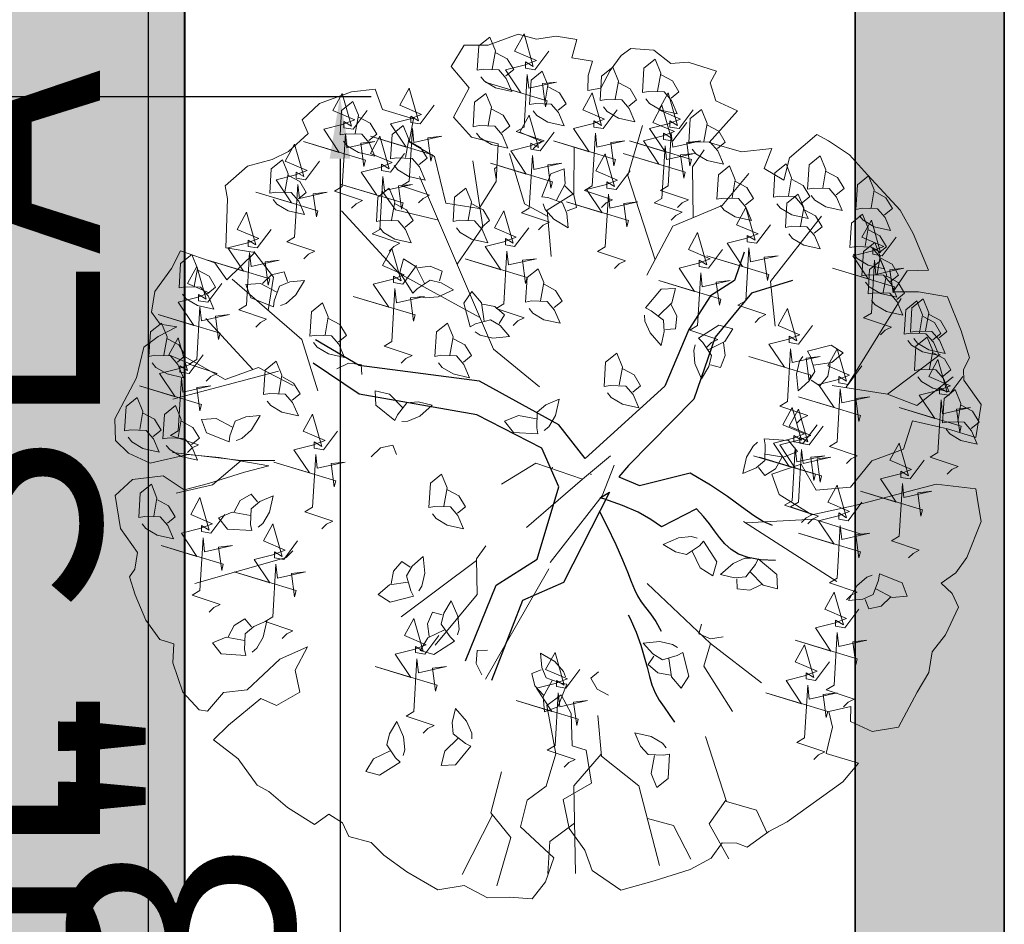
# Model space of a CAD drawing. Units: inches. Extents: x 2337 to 3570, y 1258 to 1938.
# Tile 16 of 30: x 2866 to 2906, y 1722 to 1758. Entities that reach past the tile are written whole.
import ezdxf

# ---------------------------------------------------------------- set-up
doc = ezdxf.new("R2010")
doc.units = ezdxf.units.IN
for name, color, linetype, lineweight in [('A-ANNO-DIMS', 2, 'Continuous', 18), ('A-WALL', 7, 'Continuous', 40), ('ARBOL', 74, 'Continuous', 13), ('C-PROP', 7, 'Continuous', 35)]:
    doc.layers.add(name, color=color, linetype=linetype, lineweight=lineweight)
doc.layers.add('A-WALL-PATT', color=18, linetype='Continuous', lineweight=13, true_color=0x000000)
doc.layers.add('C-PROP-PATT', color=251, linetype='Continuous', lineweight=13, true_color=0x636466)
doc.layers.add('TALLO', color=36, linetype='Continuous')
doc.styles.get("Standard").update_dxf_attribs({"font": 'arial.ttf'})
doc.dimstyles.new('ISO-25', dxfattribs={"dimtxt": 9, "dimasz": 2.5, "dimexe": 1.25, "dimexo": 0.625, "dimtad": 1, "dimdec": 1, "dimlunit": 3, "dimtxsty": 'Standard', "dimcen": 2.5, "dimadec": 0, "dimazin": 0, "dimtfac": 1, "dimtdec": 1, "dimtmove": 0, "dimatfit": 3, "dimfxl": 1, "dimarcsym": 0})

# ---------------------------------------------------------------- blocks, each defined once
blk = doc.blocks.new('fresno')
at = {"layer": 'ARBOL'}
for p, q in [((2.96, 0.991), (3.575, 1.984)), ((-3.638, 1.194), (-4.164, 1.76)), ((-1.151, -0.932), (-1.99, -1.556)), ((-0.974, -3.757), (-1.31, -4.423))]:
    blk.add_line(p, q, dxfattribs=at)
blk.add_lwpolyline([(0.823, 4.745), (0.566, 4.764), (0.459, 4.687), (0.336, 4.518), (0.233, 4.322), (0.087, 4.298), (0.091, 4.464), (0.14, 4.621), (-0.09, 4.659), (-0.033, 4.863), (-0.264, 4.901), (-0.483, 4.866), (-0.686, 4.924), (-1.021, 4.801), (-1.288, 4.8), (-1.431, 4.563), (-1.234, 4.327), (-1.406, 4), (-1.205, 3.778), (-0.909, 3.705), (-0.931, 3.283), (-1.122, 2.983), (-1.491, 3.043), (-1.619, 3.562), (-1.9, 3.727), (-1.851, 3.982), (-2.197, 4.084), (-2.278, 4.31), (-2.543, 4.283), (-2.896, 4.152), (-3.091, 3.971), (-3.022, 3.817), (-3.244, 3.617), (-3.424, 3.528), (-3.697, 3.455), (-3.946, 3.236), (-3.922, 3.09), (-3.94, 2.548), (-3.617, 2.495), (-3.927, 2.19), (-4.062, 2.379), (-4.443, 2.512), (-4.546, 2.316), (-4.73, 2.062), (-4.767, 1.832), (-4.671, 1.698), (-4.486, 1.667), (-4.693, 1.559), (-4.854, 1.444), (-4.934, 1.102), (-5.037, 0.905), (-5.175, 0.644), (-5.166, 0.406), (-5.024, 0.264), (-4.781, 0.153), (-4.363, 0.249), (-4.014, 0.215), (-3.783, 0.177), (-3.46, 0.124), (-3.733, 0.051), (-4.132, -0.073), (-4.404, -0.146), (-4.639, 0.011), (-4.977, -0.028), (-5.172, -0.209), (-5.113, -0.574), (-4.921, -0.843), (-4.951, -1.027), (-5.012, -1.112), (-4.95, -1.311), (-4.83, -1.592), (-4.676, -1.807), (-4.518, -1.856), (-4.529, -2.068), (-4.417, -2.394), (-4.236, -2.59), (-4.143, -2.605), (-3.967, -2.397), (-3.703, -2.37), (-3.339, -2.027), (-3.032, -1.889), (-3.169, -2.15), (-3.115, -2.396), (-3.376, -2.542), (-3.552, -2.466), (-3.909, -2.762), (-4.077, -2.924), (-3.804, -3.135), (-3.592, -3.43), (-3.461, -3.499), (-3.253, -3.676), (-2.953, -3.867), (-2.792, -3.752), (-2.642, -3.848), (-2.572, -4.001), (-2.323, -4.066), (-2.18, -4.208), (-1.926, -4.392), (-1.58, -4.591), (-1.288, -4.545), (-1.027, -4.683), (-0.788, -4.675), (-0.531, -4.693), (-0.382, -4.505), (-0.29, -4.236), (-0.66, -3.891), (-0.588, -3.595), (-0.374, -3.441), (-0.267, -3.079), (-0.368, -2.541), (-0.208, -2.426), (-0.099, -2.633), (-0.087, -2.991), (0.071, -3.04), (0.129, -3.405), (-0.185, -3.59), (-0.119, -3.909), (0.055, -4.151), (0.136, -4.377), (0.456, -4.596), (0.828, -4.491), (1.227, -4.368), (1.461, -4.241), (1.583, -4.071), (1.748, -4.075), (1.86, -4.117), (2.101, -3.944), (2.308, -3.836), (2.925, -3.393), (3.101, -3.185), (2.74, -3.078), (2.812, -2.782), (2.769, -2.61), (3.015, -2.555), (3.012, -2.721), (3.254, -2.832), (3.546, -2.785), (3.752, -2.393), (3.882, -2.177), (3.92, -1.947), (4.069, -1.758), (4.214, -1.451), (4.144, -1.297), (4.021, -1.182), (4.182, -1.067), (4.304, -0.897), (4.464, -0.497), (4.429, -0.279), (4.406, -0.133), (3.964, -0.083), (3.074, -0.315), (2.582, -0.424), (2.217, -0.197), (2.136, 0.029), (2.462, 0.141), (2.628, -0.147), (3.012, -0.116), (3.249, 0.177), (3.602, 0.308), (3.701, 0.623), (4.089, 0.535), (4.404, 0.436), (4.464, 0.805), (4.272, 1.074), (4.267, 1.193), (4.336, 1.324), (4.243, 1.623), (4.092, 2.003), (3.769, 2.057), (3.485, 2.056), (3.642, 2.291), (3.88, 2.299), (3.71, 2.706), (3.563, 2.967), (3.201, 3.358), (3.001, 3.581), (2.766, 3.738), (2.635, 3.807), (2.332, 3.549), (2.268, 3.299), (2.052, 3.429), (2.136, 3.652), (1.798, 3.613), (1.437, 3.72), (1.755, 4.071), (1.513, 4.182), (1.451, 4.381), (1.519, 4.512), (1.204, 4.611), (1.012, 4.596)], close=True, dxfattribs=at)
for points in [[(-1.104, 4.45), (-1.063, 4.399), (-0.939, 4.325), (-0.757, 4.285), (-0.82, 4.431), (-0.903, 4.527), (-1.075, 4.533), (-1.143, 4.521), (-1.126, 4.792), (-1.002, 4.891), (-0.939, 4.738), (-0.975, 4.535)], [(-0.346, 4.735), (-0.501, 4.528), (-0.605, 4.545), (-0.605, 4.614), (-0.519, 4.563), (-0.622, 4.925), (-0.726, 4.735), (-0.484, 4.632), (-0.622, 4.58), (-0.829, 4.528), (-0.657, 4.27), (-1.053, 4.39), (-0.363, 4.183), (-0.381, 4.114), (-0.415, 4.373), (-0.26, 4.39), (-0.57, 4.321), (-0.588, 4.476), (-0.622, 3.89), (-0.708, 3.839), (-0.398, 3.735), (-0.467, 3.701), (-0.519, 3.649)], [(-0.935, 4.717), (-0.809, 4.65), (-0.736, 4.529), (-0.824, 4.459)], [(0.734, 4.203), (0.775, 4.152), (0.9, 4.078), (1.082, 4.038), (1.018, 4.185), (0.936, 4.281), (0.763, 4.287), (0.696, 4.274), (0.712, 4.546), (0.837, 4.645), (0.899, 4.491), (0.863, 4.289)], [(-0.521, 4.069), (-0.48, 4.018), (-0.356, 3.944), (-0.174, 3.904), (-0.237, 4.051), (-0.32, 4.146), (-0.492, 4.152), (-0.56, 4.14), (-0.543, 4.411), (-0.419, 4.511), (-0.356, 4.357), (-0.392, 4.154)], [(0.263, 4.114), (0.304, 4.063), (0.429, 3.989), (0.611, 3.948), (0.547, 4.095), (0.465, 4.191), (0.293, 4.197), (0.225, 4.185), (0.242, 4.456), (0.366, 4.555), (0.428, 4.402), (0.393, 4.199)], [(0.904, 4.471), (1.029, 4.404), (1.102, 4.282), (1.015, 4.212)], [(-1.623, 4.132), (-1.778, 3.925), (-1.882, 3.942), (-1.882, 4.011), (-1.795, 3.959), (-1.899, 4.321), (-2.002, 4.132), (-1.761, 4.028), (-1.899, 3.977), (-2.106, 3.925), (-1.933, 3.666), (-2.33, 3.787), (-1.64, 3.58), (-1.657, 3.511), (-1.692, 3.77), (-1.537, 3.787), (-1.847, 3.718), (-1.864, 3.873), (-1.899, 3.287), (-1.985, 3.235), (-1.675, 3.132), (-1.744, 3.097), (-1.795, 3.046)], [(-0.352, 4.337), (-0.226, 4.269), (-0.153, 4.148), (-0.241, 4.078)], [(0.433, 4.381), (0.558, 4.314), (0.631, 4.193), (0.544, 4.122)], [(-2.368, 4.073), (-2.523, 3.866), (-2.627, 3.883), (-2.627, 3.952), (-2.541, 3.9), (-2.644, 4.262), (-2.748, 4.073), (-2.506, 3.969), (-2.644, 3.918), (-2.851, 3.866), (-2.679, 3.607), (-3.075, 3.728), (-2.385, 3.521), (-2.403, 3.452), (-2.437, 3.711), (-2.282, 3.728), (-2.592, 3.659), (-2.61, 3.814), (-2.644, 3.228), (-2.73, 3.176), (-2.42, 3.073), (-2.489, 3.038), (-2.541, 2.987)], [(-2.629, 3.733), (-2.588, 3.682), (-2.463, 3.608), (-2.281, 3.568), (-2.345, 3.715), (-2.427, 3.81), (-2.6, 3.816), (-2.667, 3.804), (-2.651, 4.075), (-2.526, 4.175), (-2.464, 4.021), (-2.5, 3.818)], [(-1.149, 3.822), (-1.108, 3.771), (-0.983, 3.697), (-0.802, 3.657), (-0.865, 3.804), (-0.948, 3.9), (-1.12, 3.906), (-1.188, 3.893), (-1.171, 4.165), (-1.047, 4.264), (-0.984, 4.111), (-1.02, 3.908)], [(0.413, 4.08), (0.258, 3.873), (0.154, 3.89), (0.154, 3.959), (0.241, 3.908), (0.137, 4.27), (0.034, 4.08), (0.275, 3.977), (0.137, 3.925), (-0.07, 3.873), (0.103, 3.614), (-0.294, 3.735), (0.396, 3.528), (0.379, 3.459), (0.344, 3.718), (0.499, 3.735), (0.189, 3.666), (0.172, 3.821), (0.137, 3.235), (0.051, 3.183), (0.361, 3.08), (0.292, 3.046), (0.241, 2.994)], [(1.259, 4.08), (1.103, 3.873), (1, 3.89), (1, 3.959), (1.086, 3.908), (0.982, 4.27), (0.879, 4.08), (1.12, 3.977), (0.982, 3.925), (0.775, 3.873), (0.948, 3.614), (0.551, 3.735), (1.241, 3.528), (1.224, 3.459), (1.189, 3.718), (1.345, 3.735), (1.034, 3.666), (1.017, 3.821), (0.982, 3.235), (0.896, 3.183), (1.207, 3.08), (1.138, 3.046), (1.086, 2.994)], [(-0.98, 4.09), (-0.854, 4.023), (-0.781, 3.901), (-0.869, 3.831)], [(1.189, 3.942), (1.034, 3.735), (0.931, 3.752), (0.931, 3.821), (1.017, 3.77), (0.913, 4.132), (0.81, 3.942), (1.051, 3.839), (0.913, 3.787), (0.706, 3.735), (0.879, 3.477), (0.482, 3.597), (1.172, 3.39), (1.155, 3.321), (1.12, 3.58), (1.276, 3.597), (0.965, 3.528), (0.948, 3.683), (0.913, 3.097), (0.827, 3.046), (1.138, 2.942), (1.069, 2.908), (1.017, 2.856)], [(1.25, 3.643), (1.291, 3.592), (1.416, 3.518), (1.597, 3.478), (1.534, 3.625), (1.451, 3.721), (1.279, 3.727), (1.211, 3.714), (1.228, 3.985), (1.352, 4.085), (1.415, 3.931), (1.379, 3.729)], [(-2.459, 4), (-2.334, 3.933), (-2.261, 3.812), (-2.348, 3.742)], [(-0.287, 3.833), (-0.442, 3.626), (-0.546, 3.643), (-0.546, 3.712), (-0.46, 3.661), (-0.563, 4.023), (-0.667, 3.833), (-0.425, 3.73), (-0.563, 3.678), (-0.77, 3.626), (-0.598, 3.367), (-0.995, 3.488), (-0.304, 3.281), (-0.322, 3.212), (-0.356, 3.471), (-0.201, 3.488), (-0.511, 3.419), (-0.529, 3.574), (-0.563, 2.988), (-0.649, 2.936), (-0.339, 2.833), (-0.408, 2.799), (-0.46, 2.747)], [(-2.068, 3.464), (-2.027, 3.413), (-1.903, 3.339), (-1.721, 3.299), (-1.784, 3.446), (-1.867, 3.542), (-2.039, 3.547), (-2.107, 3.535), (-2.09, 3.806), (-1.966, 3.906), (-1.903, 3.752), (-1.939, 3.55)], [(0.837, 2.414), (0.533, 3.352), (0.697, 3.906)], [(1.419, 3.911), (1.545, 3.844), (1.618, 3.722), (1.53, 3.652)], [(-1.951, 3.597), (-2.106, 3.39), (-2.209, 3.408), (-2.209, 3.477), (-2.123, 3.425), (-2.227, 3.787), (-2.33, 3.597), (-2.089, 3.494), (-2.227, 3.442), (-2.434, 3.39), (-2.261, 3.132), (-2.658, 3.252), (-1.968, 3.046), (-1.985, 2.977), (-2.02, 3.235), (-1.864, 3.252), (-2.175, 3.183), (-2.192, 3.339), (-2.227, 2.752), (-2.313, 2.701), (-2.002, 2.597), (-2.071, 2.563), (-2.123, 2.511)], [(-1.899, 3.732), (-1.773, 3.664), (-1.7, 3.543), (-1.788, 3.473)], [(-2.898, 3.511), (-3.053, 3.304), (-3.157, 3.321), (-3.157, 3.39), (-3.071, 3.339), (-3.174, 3.701), (-3.278, 3.511), (-3.036, 3.408), (-3.174, 3.356), (-3.381, 3.304), (-3.209, 3.046), (-3.605, 3.166), (-2.915, 2.959), (-2.932, 2.89), (-2.967, 3.149), (-2.812, 3.166), (-3.122, 3.097), (-3.14, 3.253), (-3.174, 2.666), (-3.26, 2.615), (-2.95, 2.511), (-3.019, 2.477), (-3.071, 2.425)], [(-0.063, 3.671), (-0.069, 3.151), (-0.364, 2.965), (-0.319, 2.449)], [(1.259, 2.882), (1.254, 3.446), (1.381, 3.636)], [(-3.413, 3.083), (-3.373, 3.032), (-3.248, 2.958), (-3.066, 2.918), (-3.129, 3.065), (-3.212, 3.161), (-3.384, 3.167), (-3.452, 3.154), (-3.435, 3.425), (-3.311, 3.525), (-3.248, 3.371), (-3.284, 3.169)], [(-1.367, 2.367), (-1.081, 2.78), (-1.193, 3.514)], [(-0.358, 2.895), (-0.615, 3.037), (-0.783, 3.596)], [(0.558, 3.402), (0.403, 3.195), (0.299, 3.212), (0.299, 3.281), (0.386, 3.23), (0.282, 3.592), (0.179, 3.402), (0.42, 3.299), (0.282, 3.247), (0.075, 3.195), (0.248, 2.936), (-0.149, 3.057), (0.541, 2.85), (0.524, 2.781), (0.489, 3.04), (0.644, 3.057), (0.334, 2.988), (0.317, 3.143), (0.282, 2.557), (0.196, 2.505), (0.506, 2.402), (0.437, 2.368), (0.386, 2.316)], [(2.573, 3.128), (2.613, 3.077), (2.738, 3.003), (2.92, 2.963), (2.857, 3.11), (2.774, 3.205), (2.602, 3.211), (2.534, 3.199), (2.551, 3.47), (2.675, 3.57), (2.738, 3.416), (2.702, 3.214)], [(-0.923, 3.449), (-0.951, 3.425), (-0.93, 3.313)], [(-0.41, 3.035), (-0.387, 2.974), (-0.291, 2.865), (-0.131, 2.771), (-0.146, 2.93), (-0.195, 3.047), (-0.357, 3.106), (-0.425, 3.115), (-0.325, 3.368), (-0.176, 3.424), (-0.164, 3.258), (-0.261, 3.077)], [(1.564, 3.016), (1.605, 2.965), (1.729, 2.891), (1.911, 2.851), (1.848, 2.998), (1.765, 3.094), (1.593, 3.099), (1.525, 3.087), (1.542, 3.358), (1.666, 3.458), (1.729, 3.304), (1.693, 3.102)], [(2.191, 3.038), (2.232, 2.987), (2.357, 2.913), (2.539, 2.873), (2.475, 3.02), (2.393, 3.116), (2.221, 3.122), (2.153, 3.109), (2.17, 3.381), (2.294, 3.48), (2.356, 3.326), (2.321, 3.124)], [(-3.244, 3.351), (-3.118, 3.284), (-3.045, 3.162), (-3.133, 3.092)], [(-0.448, 1), (-0.961, 1.419), (-1.784, 3.341)], [(0.746, 2.242), (1.034, 2.786), (1.584, 3.019), (1.879, 3.374)], [(2.361, 3.306), (2.486, 3.239), (2.559, 3.117), (2.472, 3.047)], [(2.742, 3.396), (2.868, 3.328), (2.941, 3.207), (2.853, 3.137)], [(3.111, 2.904), (3.152, 2.853), (3.276, 2.779), (3.458, 2.739), (3.395, 2.886), (3.312, 2.981), (3.14, 2.987), (3.072, 2.975), (3.089, 3.246), (3.213, 3.346), (3.276, 3.192), (3.24, 2.99)], [(-2.225, 2.77), (-2.184, 2.718), (-2.06, 2.645), (-1.878, 2.604), (-1.941, 2.751), (-2.024, 2.847), (-2.196, 2.853), (-2.264, 2.84), (-2.247, 3.112), (-2.123, 3.211), (-2.06, 3.058), (-2.096, 2.855)], [(-1.575, 2.854), (-2.052, 2.969), (-2.2, 3.178)], [(-1.373, 2.77), (-1.332, 2.718), (-1.208, 2.645), (-1.026, 2.604), (-1.089, 2.751), (-1.172, 2.847), (-1.344, 2.853), (-1.412, 2.84), (-1.395, 3.112), (-1.271, 3.211), (-1.208, 3.058), (-1.244, 2.855)], [(-0.166, 3.238), (-0.068, 3.135), (-0.036, 2.997), (-0.141, 2.957)], [(1.733, 3.284), (1.859, 3.216), (1.932, 3.095), (1.844, 3.025)], [(2.326, 2.702), (2.367, 2.651), (2.492, 2.577), (2.673, 2.537), (2.61, 2.684), (2.527, 2.78), (2.355, 2.786), (2.287, 2.773), (2.304, 3.045), (2.428, 3.144), (2.491, 2.99), (2.455, 2.788)], [(3.28, 3.172), (3.406, 3.104), (3.479, 2.983), (3.391, 2.913)], [(-2.056, 3.037), (-1.93, 2.97), (-1.857, 2.849), (-1.945, 2.778)], [(-0.57, 2.77), (-0.726, 2.563), (-0.829, 2.58), (-0.829, 2.649), (-0.743, 2.597), (-0.846, 2.959), (-0.95, 2.77), (-0.708, 2.666), (-0.846, 2.615), (-1.053, 2.563), (-0.881, 2.304), (-1.278, 2.425), (-0.588, 2.218), (-0.605, 2.149), (-0.639, 2.408), (-0.484, 2.425), (-0.795, 2.356), (-0.812, 2.511), (-0.846, 1.925), (-0.933, 1.873), (-0.622, 1.77), (-0.691, 1.735), (-0.743, 1.684)], [(-1.204, 3.037), (-1.078, 2.97), (-1.005, 2.849), (-1.093, 2.778)], [(2.121, 2.804), (1.966, 2.597), (1.862, 2.615), (1.862, 2.683), (1.949, 2.632), (1.845, 2.994), (1.742, 2.804), (1.983, 2.701), (1.845, 2.649), (1.638, 2.597), (1.811, 2.339), (1.414, 2.459), (2.104, 2.252), (2.087, 2.184), (2.052, 2.442), (2.207, 2.459), (1.897, 2.39), (1.88, 2.546), (1.845, 1.959), (1.759, 1.908), (2.069, 1.804), (2, 1.77), (1.949, 1.718)], [(2.495, 2.97), (2.621, 2.903), (2.694, 2.781), (2.606, 2.711)], [(-3.434, 2.752), (-3.59, 2.546), (-3.693, 2.563), (-3.693, 2.632), (-3.607, 2.58), (-3.71, 2.942), (-3.814, 2.752), (-3.572, 2.649), (-3.71, 2.597), (-3.917, 2.546), (-3.745, 2.287), (-4.142, 2.408), (-3.452, 2.201), (-3.469, 2.132), (-3.503, 2.39), (-3.348, 2.408), (-3.659, 2.339), (-3.676, 2.494), (-3.71, 1.908), (-3.797, 1.856), (-3.486, 1.753), (-3.555, 1.718), (-3.607, 1.666)], [(-1.112, 1.773), (-2.014, 2.265), (-2.654, 2.957)], [(2.171, 1.674), (2.121, 2.172), (2.689, 2.898)], [(3.519, 2.666), (3.363, 2.459), (3.26, 2.477), (3.26, 2.546), (3.346, 2.494), (3.243, 2.856), (3.139, 2.666), (3.381, 2.563), (3.243, 2.511), (3.036, 2.459), (3.208, 2.201), (2.811, 2.321), (3.501, 2.115), (3.484, 2.046), (3.45, 2.304), (3.605, 2.321), (3.294, 2.252), (3.277, 2.408), (3.243, 1.821), (3.156, 1.77), (3.467, 1.666), (3.398, 1.632), (3.346, 1.58)], [(3.043, 2.478), (3.084, 2.427), (3.209, 2.353), (3.391, 2.313), (3.327, 2.46), (3.245, 2.556), (3.073, 2.562), (3.005, 2.549), (3.022, 2.82), (3.146, 2.92), (3.208, 2.766), (3.173, 2.564)], [(3.213, 2.746), (3.338, 2.679), (3.411, 2.557), (3.324, 2.487)], [(1.586, 2.528), (1.431, 2.321), (1.327, 2.339), (1.327, 2.408), (1.414, 2.356), (1.31, 2.718), (1.207, 2.528), (1.448, 2.425), (1.31, 2.373), (1.103, 2.321), (1.276, 2.063), (0.879, 2.184), (1.569, 1.977), (1.552, 1.908), (1.517, 2.166), (1.673, 2.184), (1.362, 2.115), (1.345, 2.27), (1.31, 1.684), (1.224, 1.632), (1.535, 1.528), (1.466, 1.494), (1.414, 1.442)], [(-1.817, 2.351), (-1.972, 2.144), (-2.075, 2.162), (-2.075, 2.231), (-1.989, 2.179), (-2.093, 2.541), (-2.196, 2.351), (-1.955, 2.248), (-2.093, 2.196), (-2.3, 2.144), (-2.127, 1.886), (-2.524, 2.006), (-1.834, 1.8), (-1.851, 1.731), (-1.886, 1.989), (-1.73, 2.006), (-2.041, 1.937), (-2.058, 2.093), (-2.093, 1.506), (-2.179, 1.455), (-1.868, 1.351), (-1.937, 1.317), (-1.989, 1.265)], [(3.178, 2.165), (3.219, 2.113), (3.344, 2.04), (3.525, 1.999), (3.462, 2.146), (3.379, 2.242), (3.207, 2.248), (3.139, 2.236), (3.156, 2.507), (3.28, 2.606), (3.343, 2.453), (3.307, 2.25)], [(-4.422, 2.03), (-4.381, 1.979), (-4.257, 1.905), (-4.075, 1.865), (-4.138, 2.012), (-4.221, 2.108), (-4.393, 2.114), (-4.461, 2.101), (-4.444, 2.372), (-4.32, 2.472), (-4.257, 2.318), (-4.293, 2.116)], [(-3.468, 1.85), (-3.409, 2.222), (-3.628, 2.505)], [(-1.786, 2.007), (-1.722, 1.99), (-1.578, 2.003), (-1.407, 2.078), (-1.545, 2.159), (-1.668, 2.188), (-1.811, 2.092), (-1.859, 2.042), (-2.004, 2.271), (-1.962, 2.425), (-1.821, 2.337), (-1.731, 2.152)], [(3.347, 2.432), (3.473, 2.365), (3.546, 2.244), (3.458, 2.173)], [(-3.986, 2.149), (-4.142, 1.942), (-4.245, 1.959), (-4.245, 2.028), (-4.159, 1.977), (-4.262, 2.339), (-4.366, 2.149), (-4.124, 2.046), (-4.262, 1.994), (-4.47, 1.942), (-4.297, 1.684), (-4.694, 1.804), (-4.004, 1.597), (-4.021, 1.528), (-4.055, 1.787), (-3.9, 1.804), (-4.211, 1.735), (-4.228, 1.89), (-4.262, 1.304), (-4.349, 1.253), (-4.038, 1.149), (-4.107, 1.115), (-4.159, 1.063)], [(-1.806, 2.323), (-1.665, 2.343), (-1.534, 2.287), (-1.564, 2.179)], [(-0.566, 1.873), (-0.525, 1.822), (-0.4, 1.748), (-0.219, 1.708), (-0.282, 1.855), (-0.365, 1.951), (-0.537, 1.957), (-0.605, 1.944), (-0.588, 2.216), (-0.464, 2.315), (-0.401, 2.162), (-0.437, 1.959)], [(3.245, 1.963), (3.286, 1.912), (3.411, 1.838), (3.593, 1.798), (3.529, 1.945), (3.447, 2.041), (3.274, 2.046), (3.206, 2.034), (3.223, 2.305), (3.347, 2.405), (3.41, 2.251), (3.374, 2.049)], [(-4.253, 2.298), (-4.127, 2.231), (-4.054, 2.109), (-4.142, 2.039)], [(-2.916, 0.958), (-3.096, 1.528), (-3.871, 2.197)], [(-3.533, 2.149), (-3.43, 2.247), (-3.292, 2.279), (-3.252, 2.174)], [(3.415, 2.231), (3.54, 2.163), (3.613, 2.042), (3.525, 1.972)], [(-3.331, 1.905), (-3.269, 1.928), (-3.161, 2.024), (-3.066, 2.184), (-3.226, 2.169), (-3.342, 2.121), (-3.401, 1.958), (-3.41, 1.89), (-3.663, 1.99), (-3.719, 2.139), (-3.554, 2.151), (-3.372, 2.054)], [(-0.397, 2.141), (-0.271, 2.074), (-0.198, 1.952), (-0.286, 1.882)], [(0.72, 1.798), (0.723, 1.733), (0.781, 1.6), (0.904, 1.46), (0.939, 1.616), (0.929, 1.742), (0.793, 1.848), (0.73, 1.878), (0.904, 2.088), (1.062, 2.095), (1.023, 1.934), (0.875, 1.791)], [(-1.164, 1.612), (-1.109, 1.576), (-0.967, 1.544), (-0.782, 1.562), (-0.888, 1.682), (-0.996, 1.748), (-1.162, 1.7), (-1.222, 1.667), (-1.29, 1.93), (-1.203, 2.063), (-1.096, 1.937), (-1.067, 1.733)], [(3.716, 1.537), (3.757, 1.486), (3.882, 1.412), (4.063, 1.372), (4, 1.519), (3.917, 1.615), (3.745, 1.621), (3.677, 1.608), (3.694, 1.88), (3.818, 1.979), (3.881, 1.825), (3.845, 1.623)], [(-2.965, 1.493), (-2.924, 1.441), (-2.799, 1.368), (-2.618, 1.327), (-2.681, 1.474), (-2.764, 1.57), (-2.936, 1.576), (-3.004, 1.564), (-2.987, 1.835), (-2.863, 1.934), (-2.8, 1.781), (-2.836, 1.578)], [(-1.085, 1.919), (-0.945, 1.893), (-0.838, 1.801), (-0.9, 1.707)], [(1.014, 1.915), (1.077, 1.787), (1.064, 1.646), (0.952, 1.64)], [(2.587, 1.684), (2.432, 1.477), (2.328, 1.494), (2.328, 1.563), (2.414, 1.511), (2.311, 1.873), (2.207, 1.684), (2.449, 1.58), (2.311, 1.528), (2.104, 1.477), (2.276, 1.218), (1.88, 1.339), (2.57, 1.132), (2.552, 1.063), (2.518, 1.321), (2.673, 1.339), (2.363, 1.27), (2.345, 1.425), (2.311, 0.839), (2.225, 0.787), (2.535, 0.684), (2.466, 0.649), (2.414, 0.597)], [(3.649, 1.515), (3.69, 1.464), (3.814, 1.39), (3.996, 1.35), (3.933, 1.497), (3.85, 1.592), (3.678, 1.598), (3.61, 1.586), (3.627, 1.857), (3.751, 1.957), (3.814, 1.803), (3.778, 1.601)], [(-2.796, 1.76), (-2.67, 1.693), (-2.597, 1.572), (-2.685, 1.501)], [(3.818, 1.783), (3.944, 1.715), (4.017, 1.594), (3.929, 1.524)], [(3.885, 1.805), (4.011, 1.738), (4.084, 1.616), (3.996, 1.546)], [(-4.759, 1.269), (-4.718, 1.217), (-4.593, 1.144), (-4.411, 1.103), (-4.475, 1.25), (-4.557, 1.346), (-4.729, 1.352), (-4.797, 1.339), (-4.78, 1.611), (-4.656, 1.71), (-4.594, 1.557), (-4.629, 1.354)], [(-1.575, 1.269), (-1.534, 1.217), (-1.409, 1.144), (-1.228, 1.103), (-1.291, 1.25), (-1.373, 1.346), (-1.546, 1.352), (-1.614, 1.339), (-1.597, 1.611), (-1.473, 1.71), (-1.41, 1.557), (-1.446, 1.354)], [(1.283, 1.469), (1.266, 1.405), (1.279, 1.261), (1.354, 1.09), (1.435, 1.228), (1.464, 1.351), (1.368, 1.494), (1.318, 1.542), (1.547, 1.687), (1.7, 1.645), (1.613, 1.504), (1.428, 1.414)], [(-4.193, 1.356), (-4.349, 1.149), (-4.452, 1.166), (-4.452, 1.235), (-4.366, 1.184), (-4.469, 1.546), (-4.573, 1.356), (-4.331, 1.253), (-4.469, 1.201), (-4.677, 1.149), (-4.504, 0.89), (-4.901, 1.011), (-4.211, 0.804), (-4.228, 0.735), (-4.262, 0.994), (-4.107, 1.011), (-4.418, 0.942), (-4.435, 1.097), (-4.469, 0.511), (-4.556, 0.459), (-4.245, 0.356), (-4.314, 0.322), (-4.366, 0.27)], [(-4.589, 1.536), (-4.464, 1.469), (-4.391, 1.348), (-4.478, 1.277)], [(-1.406, 1.536), (-1.28, 1.469), (-1.207, 1.348), (-1.295, 1.277)], [(3.761, 1.112), (3.802, 1.061), (3.926, 0.987), (4.108, 0.947), (4.045, 1.093), (3.962, 1.189), (3.79, 1.195), (3.722, 1.183), (3.739, 1.454), (3.863, 1.553), (3.926, 1.4), (3.89, 1.197)], [(1.599, 1.489), (1.618, 1.348), (1.563, 1.217), (1.455, 1.247)], [(2.479, 1.34), (2.443, 1.285), (2.411, 1.143), (2.429, 0.958), (2.549, 1.064), (2.615, 1.172), (2.567, 1.338), (2.534, 1.398), (2.797, 1.466), (2.93, 1.379), (2.804, 1.272), (2.6, 1.243)], [(3.139, 1.235), (2.984, 1.028), (2.88, 1.046), (2.88, 1.115), (2.967, 1.063), (2.863, 1.425), (2.759, 1.235), (3.001, 1.132), (2.863, 1.08), (2.656, 1.028), (2.828, 0.77), (2.432, 0.891), (3.122, 0.684), (3.105, 0.615), (3.07, 0.873), (3.225, 0.891), (2.915, 0.822), (2.897, 0.977), (2.863, 0.391), (2.777, 0.339), (3.087, 0.235), (3.018, 0.201), (2.967, 0.149)], [(-3.192, 1.017), (-3.578, 1.215), (-3.949, 1.081), (-4.398, 1.339)], [(0.308, 0.933), (0.349, 0.881), (0.474, 0.807), (0.656, 0.767), (0.592, 0.914), (0.51, 1.01), (0.337, 1.016), (0.27, 1.003), (0.286, 1.275), (0.411, 1.374), (0.473, 1.221), (0.437, 1.018)], [(4.01, 1.36), (3.422, 0.918)], [(3.93, 1.379), (4.056, 1.312), (4.129, 1.191), (4.041, 1.121)], [(-3.481, 0.843), (-3.44, 0.792), (-3.315, 0.718), (-3.133, 0.678), (-3.197, 0.825), (-3.279, 0.92), (-3.451, 0.926), (-3.519, 0.914), (-3.502, 1.185), (-3.378, 1.285), (-3.316, 1.131), (-3.351, 0.928)], [(-2.703, 1.201), (-2.575, 1.263), (-2.433, 1.251), (-2.428, 1.139)], [(2.786, 1.261), (2.76, 1.121), (2.668, 1.014), (2.574, 1.076)], [(4.26, 1.115), (4.105, 0.908), (4.002, 0.925), (4.002, 0.994), (4.088, 0.942), (3.984, 1.304), (3.881, 1.115), (4.122, 1.011), (3.984, 0.959), (3.777, 0.908), (3.95, 0.649), (3.553, 0.77), (4.243, 0.563), (4.226, 0.494), (4.191, 0.753), (4.347, 0.77), (4.036, 0.701), (4.019, 0.856), (3.984, 0.27), (3.898, 0.218), (4.209, 0.115), (4.14, 0.08), (4.088, 0.029)], [(-3.354, 1.176), (-4.529, 0.864)], [(-3.311, 1.111), (-3.186, 1.043), (-3.113, 0.922), (-3.2, 0.852)], [(0.478, 1.2), (0.603, 1.133), (0.676, 1.011), (0.589, 0.941)], [(2.808, 1.015), (3.422, 0.918), (3.422, 0.918), (3.748, 0.794), (4.154, 1.111)], [(-5.028, 0.44), (-4.987, 0.388), (-4.862, 0.315), (-4.68, 0.274), (-4.744, 0.421), (-4.826, 0.517), (-4.998, 0.523), (-5.066, 0.511), (-5.049, 0.782), (-4.925, 0.881), (-4.863, 0.728), (-4.898, 0.525)], [(-1.981, 0.615), (-1.915, 0.618), (-1.782, 0.676), (-1.643, 0.799), (-1.799, 0.834), (-1.925, 0.824), (-2.031, 0.688), (-2.061, 0.626), (-2.27, 0.799), (-2.278, 0.958), (-2.117, 0.918), (-1.974, 0.77)], [(4.075, 0.529), (4.116, 0.478), (4.24, 0.404), (4.422, 0.364), (4.359, 0.511), (4.276, 0.607), (4.104, 0.613), (4.036, 0.6), (4.053, 0.871), (4.177, 0.971), (4.24, 0.817), (4.204, 0.615)], [(-4.602, 0.35), (-4.561, 0.299), (-4.436, 0.225), (-4.254, 0.185), (-4.318, 0.332), (-4.4, 0.428), (-4.572, 0.433), (-4.64, 0.421), (-4.623, 0.692), (-4.499, 0.792), (-4.437, 0.638), (-4.472, 0.436)], [(-0.397, 0.517), (-0.346, 0.557), (-0.272, 0.682), (-0.232, 0.864), (-0.379, 0.801), (-0.474, 0.718), (-0.48, 0.546), (-0.468, 0.478), (-0.739, 0.495), (-0.838, 0.619), (-0.685, 0.682), (-0.482, 0.646)], [(2.639, 0.58), (2.483, 0.373), (2.38, 0.391), (2.38, 0.46), (2.466, 0.408), (2.363, 0.77), (2.259, 0.58), (2.501, 0.477), (2.363, 0.425), (2.156, 0.373), (2.328, 0.115), (1.931, 0.235), (2.621, 0.029), (2.604, -0.04), (2.57, 0.218), (2.725, 0.235), (2.414, 0.166), (2.397, 0.322), (2.363, -0.265), (2.276, -0.316), (2.587, -0.42), (2.518, -0.454), (2.466, -0.506)], [(4.244, 0.797), (4.37, 0.73), (4.443, 0.608), (4.355, 0.538)], [(-4.858, 0.707), (-4.733, 0.64), (-4.66, 0.519), (-4.747, 0.448)], [(-3.824, 0.404), (-3.763, 0.427), (-3.654, 0.523), (-3.559, 0.683), (-3.719, 0.668), (-3.835, 0.62), (-3.894, 0.457), (-3.903, 0.389), (-4.156, 0.489), (-4.212, 0.638), (-4.047, 0.65), (-3.865, 0.553)], [(-2.698, 0.509), (-2.854, 0.302), (-2.957, 0.319), (-2.957, 0.388), (-2.871, 0.336), (-2.974, 0.698), (-3.078, 0.509), (-2.836, 0.405), (-2.974, 0.353), (-3.182, 0.302), (-3.009, 0.043), (-3.406, 0.164), (-2.716, -0.043), (-2.733, -0.112), (-2.767, 0.147), (-2.612, 0.164), (-2.923, 0.095), (-2.94, 0.25), (-2.974, -0.336), (-3.061, -0.388), (-2.75, -0.491), (-2.819, -0.526), (-2.871, -0.577)], [(2.708, 0.563), (2.552, 0.356), (2.449, 0.373), (2.449, 0.442), (2.535, 0.391), (2.432, 0.753), (2.328, 0.563), (2.57, 0.46), (2.432, 0.408), (2.225, 0.356), (2.397, 0.097), (2, 0.218), (2.69, 0.011), (2.673, -0.058), (2.639, 0.201), (2.794, 0.218), (2.483, 0.149), (2.466, 0.304), (2.432, -0.282), (2.345, -0.334), (2.656, -0.437), (2.587, -0.471), (2.535, -0.523)], [(-4.432, 0.618), (-4.307, 0.55), (-4.234, 0.429), (-4.321, 0.359)], [(-2.322, 0.222), (-2.219, 0.321), (-2.081, 0.353), (-2.042, 0.248)], [(1.978, 0.384), (1.927, 0.343), (1.853, 0.218), (1.813, 0.036), (1.96, 0.1), (2.056, 0.182), (2.061, 0.355), (2.049, 0.422), (2.32, 0.406), (2.42, 0.281), (2.266, 0.219), (2.064, 0.254)], [(3.829, 0.184), (3.674, -0.023), (3.57, -0.006), (3.57, 0.063), (3.657, 0.011), (3.553, 0.373), (3.45, 0.184), (3.691, 0.08), (3.553, 0.029), (3.346, -0.023), (3.519, -0.282), (3.122, -0.161), (3.812, -0.368), (3.795, -0.437), (3.76, -0.178), (3.915, -0.161), (3.605, -0.23), (3.588, -0.075), (3.553, -0.661), (3.467, -0.713), (3.777, -0.816), (3.708, -0.851), (3.657, -0.902)], [(-3.394, 0.18), (-3.77, 0.182), (-4.532, 0.27)], [(-0.596, -0.564), (0.03, -0.026), (0.339, 0.235)], [(-3.77, 0.182), (-4.09, -0.088), (-4.494, -0.18)], [(0.03, -0.026), (-0.491, 0.154), (-0.871, -0.08)], [(0.38, 0.131), (0.248, -0.21), (-0.33, -0.951)], [(2.246, 0.214), (2.178, 0.089), (2.057, 0.016), (1.987, 0.103)], [(-1.642, -0.412), (-1.601, -0.463), (-1.477, -0.537), (-1.295, -0.577), (-1.358, -0.43), (-1.441, -0.334), (-1.613, -0.328), (-1.681, -0.341), (-1.664, -0.069), (-1.54, 0.03), (-1.477, -0.124), (-1.513, -0.326)], [(-4.871, -0.524), (-4.83, -0.575), (-4.705, -0.649), (-4.523, -0.689), (-4.587, -0.542), (-4.669, -0.446), (-4.841, -0.44), (-4.909, -0.453), (-4.893, -0.181), (-4.768, -0.082), (-4.706, -0.236), (-4.741, -0.438)], [(3.139, -0.282), (2.984, -0.489), (2.88, -0.471), (2.88, -0.402), (2.967, -0.454), (2.863, -0.092), (2.759, -0.282), (3.001, -0.385), (2.863, -0.437), (2.656, -0.489), (2.828, -0.747), (2.432, -0.627), (3.122, -0.834), (3.105, -0.902), (3.07, -0.644), (3.225, -0.627), (2.915, -0.696), (2.897, -0.54), (2.863, -1.127), (2.777, -1.178), (3.087, -1.282), (3.018, -1.316), (2.967, -1.368)], [(-3.58, -0.559), (-3.529, -0.518), (-3.455, -0.393), (-3.415, -0.211), (-3.562, -0.275), (-3.658, -0.357), (-3.664, -0.53), (-3.651, -0.597), (-3.923, -0.581), (-4.022, -0.456), (-3.868, -0.394), (-3.666, -0.43)], [(-3.848, -0.389), (-3.781, -0.264), (-3.659, -0.191), (-3.589, -0.278)], [(-1.473, -0.144), (-1.347, -0.211), (-1.274, -0.333), (-1.362, -0.403)], [(-4.701, -0.256), (-4.576, -0.323), (-4.503, -0.445), (-4.59, -0.515)], [(-3.952, -0.42), (-4.107, -0.627), (-4.211, -0.609), (-4.211, -0.54), (-4.124, -0.592), (-4.228, -0.23), (-4.331, -0.42), (-4.09, -0.523), (-4.228, -0.575), (-4.435, -0.627), (-4.262, -0.885), (-4.659, -0.765), (-3.969, -0.971), (-3.986, -1.04), (-4.021, -0.782), (-3.866, -0.765), (-4.176, -0.834), (-4.193, -0.678), (-4.228, -1.265), (-4.314, -1.316), (-4.004, -1.42), (-4.073, -1.454), (-4.124, -1.506)], [(-3.141, -0.713), (-3.296, -0.92), (-3.4, -0.902), (-3.4, -0.834), (-3.314, -0.885), (-3.417, -0.523), (-3.521, -0.713), (-3.279, -0.816), (-3.417, -0.868), (-3.624, -0.92), (-3.452, -1.178), (-3.848, -1.058), (-3.158, -1.265), (-3.175, -1.333), (-3.21, -1.075), (-3.055, -1.058), (-3.365, -1.127), (-3.383, -0.971), (-3.417, -1.558), (-3.503, -1.609), (-3.193, -1.713), (-3.262, -1.747), (-3.314, -1.799)], [(1.822, -0.495), (2.859, -1.165)], [(1.846, -0.51), (2.605, -0.469), (3.129, -0.637)], [(-1.047, -0.767), (-1.151, -0.913), (-1.144, -1.307), (-1.61, -1.871)], [(1.304, -0.681), (1.241, -0.664), (1.097, -0.678), (0.926, -0.752), (1.064, -0.833), (1.187, -0.862), (1.33, -0.766), (1.377, -0.716), (1.523, -0.945), (1.481, -1.099), (1.34, -1.011), (1.25, -0.826)], [(-3.195, -0.824), (-3.267, -0.898), (-4.285, -1.185)], [(-1.794, -1.268), (-1.758, -1.214), (-1.726, -1.072), (-1.744, -0.887), (-1.865, -0.993), (-1.93, -1.101), (-1.883, -1.266), (-1.85, -1.327), (-2.113, -1.395), (-2.246, -1.307), (-2.119, -1.2), (-1.916, -1.172)], [(-2.101, -1.19), (-2.076, -1.05), (-1.983, -0.943), (-1.889, -1.004)], [(1.903, -0.903), (1.837, -0.905), (1.704, -0.963), (1.565, -1.086), (1.721, -1.122), (1.847, -1.111), (1.953, -0.975), (1.983, -0.913), (2.192, -1.086), (2.2, -1.245), (2.039, -1.205), (1.896, -1.057)], [(-0.346, -1.024), (-1.05, -2.251)], [(3.253, -1.094), (3.192, -1.117), (3.083, -1.213), (2.988, -1.374), (3.148, -1.359), (3.264, -1.31), (3.323, -1.148), (3.332, -1.079), (3.585, -1.179), (3.641, -1.328), (3.476, -1.34), (3.294, -1.244)], [(0.748, -1.185), (1.452, -1.855), (2.021, -2.292)], [(2.02, -1.197), (1.891, -1.259), (1.75, -1.247), (1.745, -1.134)], [(3.105, -1.471), (2.949, -1.678), (2.846, -1.661), (2.846, -1.592), (2.932, -1.644), (2.829, -1.282), (2.725, -1.471), (2.967, -1.575), (2.829, -1.627), (2.621, -1.678), (2.794, -1.937), (2.397, -1.816), (3.087, -2.023), (3.07, -2.092), (3.036, -1.833), (3.191, -1.816), (2.88, -1.885), (2.863, -1.73), (2.829, -2.316), (2.742, -2.368), (3.053, -2.471), (2.984, -2.506), (2.932, -2.558)], [(-1.361, -1.756), (-1.343, -1.693), (-1.357, -1.548), (-1.431, -1.377), (-1.513, -1.515), (-1.542, -1.638), (-1.445, -1.781), (-1.395, -1.829), (-1.625, -1.974), (-1.778, -1.932), (-1.691, -1.791), (-1.506, -1.701)], [(3.455, -1.338), (3.352, -1.437), (3.214, -1.469), (3.175, -1.364)], [(-1.677, -1.776), (-1.696, -1.635), (-1.641, -1.504), (-1.533, -1.534)], [(-3.648, -1.948), (-3.596, -1.907), (-3.523, -1.782), (-3.482, -1.6), (-3.629, -1.664), (-3.725, -1.746), (-3.731, -1.919), (-3.719, -1.986), (-3.99, -1.97), (-4.089, -1.845), (-3.936, -1.783), (-3.733, -1.819)], [(-3.915, -1.778), (-3.848, -1.653), (-3.727, -1.58), (-3.656, -1.667)], [(-1.571, -1.764), (-1.726, -1.971), (-1.83, -1.954), (-1.83, -1.885), (-1.744, -1.937), (-1.847, -1.575), (-1.951, -1.764), (-1.709, -1.868), (-1.847, -1.92), (-2.054, -1.971), (-1.882, -2.23), (-2.278, -2.109), (-1.588, -2.316), (-1.605, -2.385), (-1.64, -2.127), (-1.485, -2.109), (-1.795, -2.178), (-1.813, -2.023), (-1.847, -2.609), (-1.933, -2.661), (-1.623, -2.764), (-1.692, -2.799), (-1.744, -2.851)], [(1.593, -1.781), (1.452, -1.801), (1.322, -1.746), (1.352, -1.637)], [(1.086, -1.899), (1.031, -1.863), (0.89, -1.831), (0.704, -1.849), (0.81, -1.969), (0.918, -2.035), (1.084, -1.987), (1.145, -1.954), (1.212, -2.218), (1.125, -2.35), (1.018, -2.224), (0.989, -2.02)], [(1.452, -1.855), (1.379, -2.105), (1.698, -2.609)], [(-1.092, -2.202), (-1.154, -2.074), (-1.142, -1.933), (-1.03, -1.928)], [(-0.001, -2.144), (-0.156, -2.351), (-0.26, -2.333), (-0.26, -2.264), (-0.174, -2.316), (-0.277, -1.954), (-0.381, -2.144), (-0.139, -2.247), (-0.277, -2.299), (-0.484, -2.351), (-0.312, -2.609), (-0.708, -2.489), (-0.018, -2.695), (-0.035, -2.764), (-0.07, -2.506), (0.085, -2.489), (-0.225, -2.558), (-0.243, -2.402), (-0.277, -2.989), (-0.363, -3.04), (-0.053, -3.144), (-0.122, -3.178), (-0.174, -3.23)], [(-0.161, -2.225), (-0.184, -2.163), (-0.28, -2.055), (-0.44, -1.96), (-0.425, -2.12), (-0.376, -2.236), (-0.214, -2.295), (-0.146, -2.304), (-0.246, -2.557), (-0.395, -2.613), (-0.407, -2.448), (-0.31, -2.266)], [(2.777, -2.058), (2.621, -2.264), (2.518, -2.247), (2.518, -2.178), (2.604, -2.23), (2.501, -1.868), (2.397, -2.058), (2.639, -2.161), (2.501, -2.213), (2.294, -2.264), (2.466, -2.523), (2.069, -2.402), (2.759, -2.609), (2.742, -2.678), (2.708, -2.42), (2.863, -2.402), (2.552, -2.471), (2.535, -2.316), (2.501, -2.902), (2.414, -2.954), (2.725, -3.057), (2.656, -3.092), (2.604, -3.144)], [(1.007, -2.206), (0.867, -2.181), (0.76, -2.088), (0.822, -1.994)], [(-0.405, -2.427), (-0.503, -2.324), (-0.535, -2.186), (-0.43, -2.146)], [(0.319, -2.428), (0.193, -2.361), (0.12, -2.239), (0.208, -2.169)], [(-1.201, -2.914), (-1.204, -2.849), (-1.262, -2.716), (-1.385, -2.576), (-1.42, -2.732), (-1.41, -2.858), (-1.274, -2.964), (-1.212, -2.994), (-1.385, -3.204), (-1.544, -3.211), (-1.504, -3.05), (-1.356, -2.907)], [(-1.966, -3.1), (-1.949, -3.037), (-1.962, -2.892), (-2.037, -2.722), (-2.118, -2.859), (-2.147, -2.982), (-2.051, -3.125), (-2.001, -3.173), (-2.23, -3.319), (-2.383, -3.277), (-2.296, -3.136), (-2.111, -3.046)], [(0.201, -2.655), (0.24, -3.105), (0.657, -3.436), (0.886, -4.322)], [(0.959, -3.012), (0.918, -2.961), (0.793, -2.887), (0.612, -2.847), (0.675, -2.994), (0.758, -3.089), (0.93, -3.095), (0.998, -3.083), (0.981, -3.354), (0.857, -3.453), (0.794, -3.3), (0.83, -3.097)], [(1.399, -2.886), (1.63, -3.612), (1.964, -3.708), (2.084, -3.964)], [(0.238, -3.084), (-0.067, -3.438), (-0.048, -4.412)], [(-0.923, -4.549), (-0.768, -4.012), (-0.99, -3.737), (-0.872, -3.28)], [(1.625, -3.596), (1.438, -3.858), (1.657, -4.248)], [(0.752, -3.801), (1.042, -3.878), (1.233, -4.25)], [(-0.059, -3.851), (-0.336, -4.054), (-0.355, -4.41)]]:
    blk.add_lwpolyline(points, dxfattribs=at)
for p in [(-0.308, 0.101), (0.124, 0.027)]:
    blk.add_point(p, dxfattribs=at)
at = {"layer": 'TALLO'}
for points in [[(1.829, 2.5), (1.722, 2.184), (1.454, 2.012), (1.213, 1.639), (0.944, 1.008), (0.06, 0.204), (-0.234, 0.577), (-1.119, 1.065), (-2.458, 1.237), (-2.941, 1.524)], [(2.364, 2.184), (1.909, 2.041), (1.507, 1.552), (1.266, 0.864), (0.542, 0.125), (0.433, 0.001), (0.662, -0.096), (1.228, 0.045), (1.455, -0.09), (1.644, -0.216), (1.8, -0.33), (1.931, -0.425), (2.042, -0.496), (2.141, -0.539)], [(-1.272, -2.047), (-0.931, -1.203), (-0.475, -0.916), (-0.234, -0.112), (-0.422, 0.318), (-1.146, 0.691), (-2.458, 0.921), (-2.967, 1.266)], [(2.177, -0.932), (2.008, -0.924), (1.873, -0.898), (1.766, -0.859), (1.682, -0.807), (1.613, -0.745), (1.554, -0.676), (1.499, -0.6), (1.442, -0.521), (1.376, -0.44), (1.298, -0.357), (0.908, -0.555), (0.791, -0.474), (0.647, -0.394), (0.474, -0.317), (0.265, -0.244), (0.226, -0.233), (0.328, -0.17), (-0.181, -1.175), (-0.637, -1.375), (-0.985, -2.265)], [(0.219, -0.386), (0.3, -0.544), (0.399, -0.753), (0.473, -0.922), (0.529, -1.057), (0.571, -1.164), (0.607, -1.251), (0.641, -1.324), (0.68, -1.389), (0.729, -1.454), (0.784, -1.525), (0.844, -1.61), (0.903, -1.717)], [(0.538, -1.536), (0.555, -1.568), (0.626, -1.728), (0.678, -1.871), (0.716, -2), (0.747, -2.115), (0.773, -2.219), (0.802, -2.314), (0.837, -2.401), (0.883, -2.483), (0.936, -2.562), (0.994, -2.642), (1.052, -2.727)]]:
    blk.add_lwpolyline(points, dxfattribs=at)
blk = doc.blocks.new('*D87')
at = {"layer": 'A-ANNO-DIMS', "color": 0, "lineweight": -2, "transparency": 16777216}
for p, q in [((2864.461, 1755.116), (2880.347, 1755.116)), ((2879.097, 1752.616), (2879.097, 1682.454)), ((2864.461, 1679.954), (2880.347, 1679.954))]:
    blk.add_line(p, q, dxfattribs=at)
at = {"layer": 'A-ANNO-DIMS', "color": 0, "transparency": 16777216}
for points in [[(2878.681, 1752.616), (2879.514, 1752.616), (2879.097, 1755.116)], [(2878.681, 1682.454), (2879.514, 1682.454), (2879.097, 1679.954)]]:
    blk.add_solid(points, dxfattribs=at)
at = {"layer": 'Defpoints', "color": 0, "transparency": 16777216}
for p in [(2863.836, 1755.116), (2863.836, 1679.954), (2879.097, 1679.954)]:
    blk.add_point(p, dxfattribs=at)
at = {"layer": 'A-ANNO-DIMS', "color": 0, "transparency": 16777216, "insert": (2873.874, 1717.535), "char_height": 9, "attachment_point": 5, "rotation": 90}
blk.add_mtext('6\'-3"', dxfattribs=at)
blk = doc.blocks.new('*D90')
at = {"layer": 'A-ANNO-DIMS', "color": 0, "lineweight": -2, "transparency": 16777216}
for p, q in [((2871.382, 1676.497), (2871.382, 1796.695)), ((2864.515, 1676.497), (2872.632, 1676.497)), ((2871.382, 1629.048), (2871.382, 1673.997)), ((2864.515, 1626.548), (2872.632, 1626.548))]:
    blk.add_line(p, q, dxfattribs=at)
at = {"layer": 'A-ANNO-DIMS', "color": 0, "transparency": 16777216}
for points in [[(2870.966, 1673.997), (2871.799, 1673.997), (2871.382, 1676.497)], [(2870.966, 1629.048), (2871.799, 1629.048), (2871.382, 1626.548)]]:
    blk.add_solid(points, dxfattribs=at)
at = {"layer": 'Defpoints', "color": 0, "transparency": 16777216}
for p in [(2863.89, 1676.497), (2871.382, 1676.497), (2863.89, 1626.548)]:
    blk.add_point(p, dxfattribs=at)
at = {"layer": 'A-ANNO-DIMS', "color": 0, "transparency": 16777216, "insert": (2866.101, 1737.846), "char_height": 9, "attachment_point": 5, "rotation": 90}
blk.add_mtext('LOUNGE SEAT 4\'-2"', dxfattribs=at)

msp = doc.modelspace()

# ---------------------------------------------------------------- hatches: boundary and pattern name
at = {"layer": 'A-WALL-PATT'}
h = msp.add_hatch(color=256, dxfattribs=at)
h.dxf.hatch_style = 1
h.paths.add_polyline_path([(2671.836, 1857.116), (2455.836, 1857.116), (2455.836, 1824.116), (2464.836, 1824.116), (2464.836, 1848.116), (2671.836, 1848.116)])
h.paths.add_polyline_path([(2566.836, 1764.116), (2464.836, 1764.116), (2464.836, 1788.116), (2455.836, 1788.116), (2455.836, 1743.116), (2464.836, 1743.116), (2464.836, 1755.116), (2566.836, 1755.116)])
h.paths.add_polyline_path([(2683.836, 1761.116), (2683.836, 1764.116), (2602.836, 1764.116), (2602.836, 1755.116), (2608.836, 1755.116), (2608.836, 1701.116), (2662.836, 1701.116), (2662.836, 1605.116), (2671.836, 1605.116), (2671.836, 1713.116), (2662.836, 1713.116), (2662.836, 1707.116), (2614.836, 1707.116), (2614.836, 1755.116), (2662.836, 1755.116), (2662.836, 1749.116), (2671.836, 1749.116), (2671.836, 1755.116), (2683.836, 1755.116)])
h.paths.add_polyline_path([(2464.836, 1707.116), (2455.836, 1707.116), (2455.836, 1617.116), (2464.836, 1617.116), (2464.836, 1635.116), (2506.836, 1635.116), (2506.836, 1641.116), (2464.836, 1641.116)])
h.paths.add_polyline_path([(2542.836, 1551.116), (2464.836, 1551.116), (2464.836, 1569.116), (2455.836, 1569.116), (2455.836, 1518.116), (2464.836, 1518.116), (2464.836, 1542.116), (2542.836, 1542.116)])
h.paths.add_polyline_path([(2464.836, 1482.116), (2455.836, 1482.116), (2455.836, 1410.116), (2464.836, 1410.116)])
h.paths.add_polyline_path([(2626.836, 1350.116), (2590.836, 1350.116), (2590.836, 1380.116), (2584.836, 1380.116), (2584.836, 1350.116), (2464.836, 1350.116), (2464.836, 1374.116), (2455.836, 1374.116), (2455.836, 1341.116), (2626.836, 1341.116)])
h.paths.add_polyline_path([(2662.836, 1416.116), (2686.836, 1416.116), (2686.836, 1422.116), (2590.836, 1422.116), (2590.836, 1542.116), (2680.836, 1542.116), (2680.836, 1551.116), (2671.836, 1551.116), (2671.836, 1557.116), (2662.836, 1557.116), (2662.836, 1551.116), (2578.836, 1551.116), (2578.836, 1542.116), (2584.836, 1542.116), (2584.836, 1410.116), (2590.836, 1410.116), (2590.836, 1416.116), (2656.836, 1416.116), (2656.836, 1350.116), (2650.836, 1350.116), (2650.836, 1341.116), (2731.836, 1341.116), (2731.836, 1362.116), (2722.836, 1362.116), (2722.836, 1350.116), (2662.836, 1350.116)])
h.paths.add_polyline_path([(2731.836, 1434.116), (2722.836, 1434.116), (2722.836, 1422.116), (2716.836, 1422.116), (2716.836, 1416.116), (2722.836, 1416.116), (2722.836, 1386.116), (2731.836, 1386.116)], flags=17)
h.paths.add_polyline_path([(2731.836, 1542.116), (2752.836, 1542.116), (2752.836, 1551.116), (2716.836, 1551.116), (2716.836, 1545.116), (2716.836, 1542.116), (2722.836, 1542.116), (2722.836, 1482.116), (2731.836, 1482.116)])
h.paths.add_polyline_path([(2809.836, 1551.116), (2788.836, 1551.116), (2788.836, 1542.116), (2809.836, 1542.116), (2809.836, 1548.116)])
h.paths.add_polyline_path([(2872.836, 1647.116), (2863.836, 1647.116), (2863.836, 1551.116), (2857.836, 1551.116), (2857.836, 1548.116), (2857.836, 1542.116), (2872.836, 1542.116)])
h.paths.add_polyline_path([(2872.836, 1764.116), (2827.836, 1764.116), (2827.836, 1755.116), (2863.836, 1755.116), (2863.836, 1719.116), (2872.836, 1719.116)])
h.paths.add_polyline_path([(2755.836, 1764.116), (2719.836, 1764.116), (2719.836, 1755.116), (2755.836, 1755.116)])
at = {"layer": 'C-PROP-PATT'}
h = msp.add_hatch(color=256, dxfattribs=at)
h.dxf.hatch_style = 1
h.paths.add_polyline_path([(2905.836, 1893.116), (2425.836, 1893.116), (2425.836, 1293.116), (2731.836, 1293.116), (2731.836, 1299.116), (2431.836, 1299.116), (2431.836, 1887.116), (2899.836, 1887.116), (2899.836, 1875.116), (2905.836, 1875.116)])
h.paths.add_polyline_path([(2845.836, 1299.116), (2827.836, 1299.116), (2827.836, 1293.116), (2845.836, 1293.116)], flags=17)
h.paths.add_polyline_path([(2905.836, 1779.116), (2899.836, 1779.116), (2899.836, 1299.116), (2893.836, 1299.116), (2893.836, 1293.116), (2905.836, 1293.116)], flags=17)

# ---------------------------------------------------------------- linework, layer by layer
at = {"layer": 'A-WALL'}
msp.add_line((2872.836, 1764.116), (2872.836, 1542.116), dxfattribs=at)
at = {"layer": 'C-PROP'}
for p, q in [((2899.836, 1779.116), (2899.836, 1299.116)), ((2905.836, 1779.116), (2905.836, 1293.116))]:
    msp.add_line(p, q, dxfattribs=at)

# ---------------------------------------------------------------- block references
at = {"layer": 'ARBOL', "xscale": 3.617267037020409, "yscale": 3.617267037020409, "zscale": 3.617267037020409}
msp.add_blockref('fresno', (2888.753, 1739.819), dxfattribs=at)

# ---------------------------------------------------------------- dimensions: what is measured, and where the dimension line sits
at = {"layer": 'A-ANNO-DIMS'}
dim = msp.add_linear_dim(base=(2871.382, 1676.497), p1=(2863.89, 1626.548), p2=(2863.89, 1676.497), angle=90, text='LOUNGE SEAT <>', dimstyle='ISO-25', override={"dimdec": 1, "dimlfac": 1, "dimrnd": 0, "dimzin": 1, "dimdsep": 46, "dimlunit": 4, "dimfrac": 2}, dxfattribs=at)
dim.commit()
dim.dimension.update_dxf_attribs({"geometry": '*D90', "text_midpoint": (2866.101, 1737.846)})
dim = msp.add_linear_dim(base=(2879.097, 1679.954), p1=(2863.836, 1755.116), p2=(2863.836, 1679.954), angle=270, dimstyle='ISO-25', override={"dimdec": 1, "dimlfac": 1, "dimrnd": 0, "dimzin": 1, "dimdsep": 46, "dimlunit": 4, "dimfrac": 2}, dxfattribs=at)
dim.commit()
dim.dimension.update_dxf_attribs({"geometry": '*D87', "text_midpoint": (2873.874, 1717.535)})

doc.saveas('drawing.dxf')
